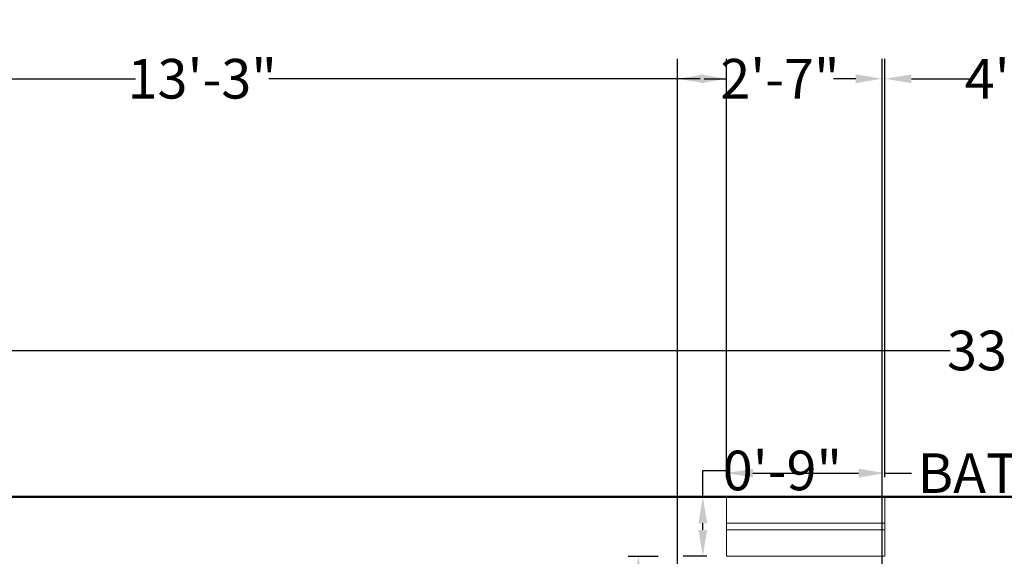
# Model space of a CAD drawing. Units: inches. Extents: x -59 to 502, y -260 to 136.
# Tile 7 of 8: x 77 to 226, y 55 to 136. Entities that reach past the tile are written whole.
import ezdxf

# ---------------------------------------------------------------- set-up
doc = ezdxf.new("R2010")
doc.units = ezdxf.units.IN
doc.header["$MEASUREMENT"] = 0
for name, color, linetype, lineweight in [('A-ANNO-DIMS', 2, 'Continuous', 18), ('Outer Wall', 10, 'Continuous', 50), ('Ventilator', 130, 'Continuous', 18)]:
    doc.layers.add(name, color=color, linetype=linetype, lineweight=lineweight)
doc.styles.get("Standard").update_dxf_attribs({"font": 'arial.ttf'})
doc.dimstyles.get("Standard").update_dxf_attribs({"dimtxt": 6, "dimasz": 4, "dimexe": 3, "dimexo": 3, "dimgap": 0.09, "dimtad": 0, "dimtih": 1, "dimtoh": 1, "dimdec": 1, "dimzin": 0, "dimdsep": 46, "dimlunit": 3, "dimtxsty": 'Standard', "dimcen": 0.09, "dimadec": 0, "dimazin": 0, "dimtfac": 1, "dimtdec": 1, "dimtofl": 0, "dimtmove": 0, "dimatfit": 3, "dimfxl": 1, "dimtolj": 1, "dimtzin": 0, "dimarcsym": 0})

# ---------------------------------------------------------------- blocks, each defined once
blk = doc.blocks.new('Ventilator (V)')
for p, q in [((947.23, 175.12), (971.23, 175.12)), ((947.23, 166.12), (947.23, 175.12)), ((971.23, 175.12), (971.23, 166.12)), ((947.23, 171.12), (971.23, 171.12)), ((971.23, 170.12), (947.23, 170.12)), ((971.23, 166.12), (947.23, 166.12))]:
    blk.add_line(p, q)
blk = doc.blocks.new('*D7')
at = {"layer": 'A-ANNO-DIMS', "color": 0, "lineweight": -2, "transparency": 16777216}
for p, q in [((25.46, 66.92), (25.46, 89.09)), ((421.46, 66.92), (421.46, 89.09)), ((29.46, 86.09), (218.28, 86.09)), ((417.46, 86.09), (228.64, 86.09))]:
    blk.add_line(p, q, dxfattribs=at)
at = {"layer": 'A-ANNO-DIMS', "color": 0, "transparency": 16777216}
for points in [[(29.46, 86.75), (29.46, 85.42), (25.46, 86.09)], [(417.46, 86.75), (417.46, 85.42), (421.46, 86.09)]]:
    blk.add_solid(points, dxfattribs=at)
at = {"layer": 'Defpoints', "color": 0, "transparency": 16777216}
for p in [(421.46, 86.09), (25.46, 63.92), (421.46, 63.92)]:
    blk.add_point(p, dxfattribs=at)
at = {"layer": 'A-ANNO-DIMS', "color": 0, "transparency": 16777216, "insert": (223.46, 86.09), "char_height": 6, "attachment_point": 5}
blk.add_mtext("\\A1;33'", dxfattribs=at)
blk = doc.blocks.new('*D33')
at = {"layer": 'A-ANNO-DIMS', "color": 0, "lineweight": -2, "transparency": 16777216}
for p, q in [((169.46, 54.92), (174.01, 54.92)), ((171.01, 50.92), (171.01, 42.94)), ((171.01, 28.57), (171.01, 36.55)), ((169.46, 24.57), (174.01, 24.57))]:
    blk.add_line(p, q, dxfattribs=at)
at = {"layer": 'A-ANNO-DIMS', "color": 0, "transparency": 16777216}
for points in [[(170.34, 50.92), (171.68, 50.92), (171.01, 54.92)], [(170.34, 28.57), (171.68, 28.57), (171.01, 24.57)]]:
    blk.add_solid(points, dxfattribs=at)
at = {"layer": 'Defpoints', "color": 0, "transparency": 16777216}
for p in [(166.46, 54.92), (171.01, 54.92), (166.46, 24.57)]:
    blk.add_point(p, dxfattribs=at)
at = {"layer": 'A-ANNO-DIMS', "color": 0, "transparency": 16777216, "insert": (171.01, 39.75), "char_height": 6, "attachment_point": 5}
blk.add_mtext('\\A1;CLOSET PANEL 2\'-6 1/2" TYP.', dxfattribs=at)
blk = doc.blocks.new('*D35')
at = {"layer": 'A-ANNO-DIMS', "color": 0, "lineweight": -2, "transparency": 16777216}
for p, q in [((184.38, 66.92), (184.38, 70.52)), ((208.38, 66.92), (208.38, 70.52)), ((188.38, 67.52), (204.38, 67.52)), ((208.38, 67.52), (212.38, 67.52))]:
    blk.add_line(p, q, dxfattribs=at)
at = {"layer": 'A-ANNO-DIMS', "color": 0, "transparency": 16777216}
for points in [[(188.38, 68.19), (188.38, 66.86), (184.38, 67.52)], [(204.38, 68.19), (204.38, 66.86), (208.38, 67.52)]]:
    blk.add_solid(points, dxfattribs=at)
at = {"layer": 'Defpoints', "color": 0, "transparency": 16777216}
for p in [(208.38, 67.52), (184.38, 63.92), (208.38, 63.92)]:
    blk.add_point(p, dxfattribs=at)
at = {"layer": 'A-ANNO-DIMS', "color": 0, "transparency": 16777216, "insert": (244.99, 67.52), "char_height": 6, "attachment_point": 5}
blk.add_mtext('\\A1;BATH VENT 2\'-0"', dxfattribs=at)
blk = doc.blocks.new('*D36')
at = {"layer": 'A-ANNO-DIMS', "color": 0, "lineweight": -2, "transparency": 16777216}
for p, q in [((180.78, 63.92), (180.78, 67.92)), ((180.78, 67.92), (184.78, 67.92)), ((181.38, 63.92), (177.78, 63.92)), ((180.78, 58.92), (180.78, 59.92)), ((181.38, 54.92), (177.78, 54.92))]:
    blk.add_line(p, q, dxfattribs=at)
at = {"layer": 'A-ANNO-DIMS', "color": 0, "transparency": 16777216}
for points in [[(180.11, 59.92), (181.44, 59.92), (180.78, 63.92)], [(180.11, 58.92), (181.44, 58.92), (180.78, 54.92)]]:
    blk.add_solid(points, dxfattribs=at)
at = {"layer": 'Defpoints', "color": 0, "transparency": 16777216}
for p in [(180.78, 63.92), (184.38, 63.92), (184.38, 54.92)]:
    blk.add_point(p, dxfattribs=at)
at = {"layer": 'A-ANNO-DIMS', "color": 0, "transparency": 16777216, "insert": (192.84, 67.92), "char_height": 6, "attachment_point": 5}
blk.add_mtext('\\A1;0\'-9"', dxfattribs=at)
blk = doc.blocks.new('*D57')
at = {"layer": 'A-ANNO-DIMS', "color": 0, "lineweight": -2, "transparency": 16777216}
for p, q in [((25.46, 66.92), (25.46, 130.25)), ((184.38, 66.92), (184.38, 130.25)), ((29.46, 127.25), (94.81, 127.25)), ((180.38, 127.25), (115.03, 127.25))]:
    blk.add_line(p, q, dxfattribs=at)
at = {"layer": 'A-ANNO-DIMS', "color": 0, "transparency": 16777216}
for points in [[(29.46, 127.91), (29.46, 126.58), (25.46, 127.25)], [(180.38, 127.91), (180.38, 126.58), (184.38, 127.25)]]:
    blk.add_solid(points, dxfattribs=at)
at = {"layer": 'Defpoints', "color": 0, "transparency": 16777216}
for p in [(184.38, 127.25), (25.46, 63.92), (184.38, 63.92)]:
    blk.add_point(p, dxfattribs=at)
at = {"layer": 'A-ANNO-DIMS', "color": 0, "transparency": 16777216, "insert": (104.92, 127.25), "char_height": 6, "attachment_point": 5}
blk.add_mtext('\\A1;13\'-3"', dxfattribs=at)
blk = doc.blocks.new('*D58')
at = {"layer": 'A-ANNO-DIMS', "color": 0, "lineweight": -2, "transparency": 16777216}
for p, q in [((208.38, 66.92), (208.38, 130.25)), ((264.77, 66.92), (264.77, 130.25)), ((212.38, 127.25), (221.4, 127.25)), ((260.77, 127.25), (251.75, 127.25))]:
    blk.add_line(p, q, dxfattribs=at)
at = {"layer": 'A-ANNO-DIMS', "color": 0, "transparency": 16777216}
for points in [[(212.38, 127.91), (212.38, 126.58), (208.38, 127.25)], [(260.77, 127.91), (260.77, 126.58), (264.77, 127.25)]]:
    blk.add_solid(points, dxfattribs=at)
at = {"layer": 'Defpoints', "color": 0, "transparency": 16777216}
for p in [(264.77, 127.25), (208.38, 63.92), (264.77, 63.92)]:
    blk.add_point(p, dxfattribs=at)
at = {"layer": 'A-ANNO-DIMS', "color": 0, "transparency": 16777216, "insert": (236.57, 127.25), "char_height": 6, "attachment_point": 5}
blk.add_mtext('\\A1;4\'-8 1/2"', dxfattribs=at)
blk = doc.blocks.new('*D69')
at = {"layer": 'A-ANNO-DIMS', "color": 0, "lineweight": -2, "transparency": 16777216}
for p, q in [((176.96, 2.92), (176.96, 130.25)), ((207.96, 2.92), (207.96, 130.25)), ((180.96, 127.25), (184.34, 127.25)), ((203.96, 127.25), (200.57, 127.25))]:
    blk.add_line(p, q, dxfattribs=at)
at = {"layer": 'A-ANNO-DIMS', "color": 0, "transparency": 16777216}
for points in [[(180.96, 127.91), (180.96, 126.58), (176.96, 127.25)], [(203.96, 127.91), (203.96, 126.58), (207.96, 127.25)]]:
    blk.add_solid(points, dxfattribs=at)
at = {"layer": 'Defpoints', "color": 0, "transparency": 16777216}
for p in [(207.96, 127.25), (176.96, -0.08), (207.96, -0.08)]:
    blk.add_point(p, dxfattribs=at)
at = {"layer": 'A-ANNO-DIMS', "color": 0, "transparency": 16777216, "insert": (192.46, 127.25), "char_height": 6, "attachment_point": 5}
blk.add_mtext('\\A1;2\'-7"', dxfattribs=at)

msp = doc.modelspace()

# ---------------------------------------------------------------- linework, layer by layer
at = {"layer": 'Outer Wall'}
msp.add_lwpolyline([(220.96, -188.08), (25.46, -188.08), (25.46, 63.92), (421.46, 63.92), (421.46, -188.08), (292.96, -188.08)], dxfattribs=at)

# ---------------------------------------------------------------- block references
at = {"layer": 'Ventilator'}
msp.add_blockref('Ventilator (V)', (-762.86, -111.2), dxfattribs=at)

# ---------------------------------------------------------------- dimensions: what is measured, and where the dimension line sits
at = {"layer": 'A-ANNO-DIMS'}
for base, p1, p2, override, picture, middle in [((264.77, 127.25), (208.38, 63.92), (264.77, 63.92), {"dimdec": 1, "dimlfac": 1, "dimrnd": 0, "dimzin": 1, "dimdsep": 46, "dimlunit": 4, "dimfrac": 2}, '*D58', (236.57, 127.25)), ((184.38, 127.25), (25.46, 63.92), (184.38, 63.92), {"dimdec": 1, "dimlfac": 1, "dimrnd": 0, "dimzin": 1, "dimdsep": 46, "dimlunit": 4, "dimfrac": 2}, '*D57', (104.92, 127.25)), ((207.96, 127.25), (176.96, -0.08), (207.96, -0.08), {"dimdec": 1, "dimlfac": 1, "dimrnd": 0, "dimzin": 1, "dimdsep": 46, "dimlunit": 4, "dimfrac": 2}, '*D69', (192.46, 127.25)), ((421.46, 86.09), (25.46, 63.92), (421.46, 63.92), {"dimclrd": 0, "dimclre": 0, "dimclrt": 0}, '*D7', (223.46, 86.09))]:
    dim = msp.add_linear_dim(base=base, p1=p1, p2=p2, dimstyle='Standard', override=override, dxfattribs=at)
    dim.commit()
    dim.dimension.update_dxf_attribs({"geometry": picture, "text_midpoint": middle})
dim = msp.add_linear_dim(base=(208.38, 67.52), p1=(184.38, 63.92), p2=(208.38, 63.92), text='BATH VENT <>', dimstyle='Standard', override={"dimdec": 1, "dimlfac": 1, "dimrnd": 0, "dimzin": 1, "dimdsep": 46, "dimlunit": 4, "dimfrac": 2}, dxfattribs=at)
dim.commit()
dim.dimension.update_dxf_attribs({"geometry": '*D35', "text_midpoint": (244.99, 67.52)})
dim = msp.add_linear_dim(base=(180.78, 63.92), p1=(184.38, 54.92), p2=(184.38, 63.92), angle=90, dimstyle='Standard', override={"dimdec": 1, "dimlfac": 1, "dimrnd": 0, "dimzin": 1, "dimdsep": 46, "dimlunit": 4, "dimfrac": 2}, dxfattribs=at)
dim.commit()
dim.dimension.update_dxf_attribs({"geometry": '*D36', "text_midpoint": (192.84, 67.92)})
dim = msp.add_linear_dim(base=(171.0112, 54.9218), p1=(166.4591, 24.5742), p2=(166.4591, 54.9218), angle=90, text='CLOSET PANEL <> TYP.', dimstyle='Standard', override={"dimdec": 1, "dimlfac": 1, "dimrnd": 0, "dimzin": 1, "dimdsep": 46, "dimlunit": 4, "dimfrac": 2}, dxfattribs=at)
dim.commit()
dim.dimension.update_dxf_attribs({"geometry": '*D33', "text_midpoint": (171.0112, 39.748)})

doc.saveas('drawing.dxf')
